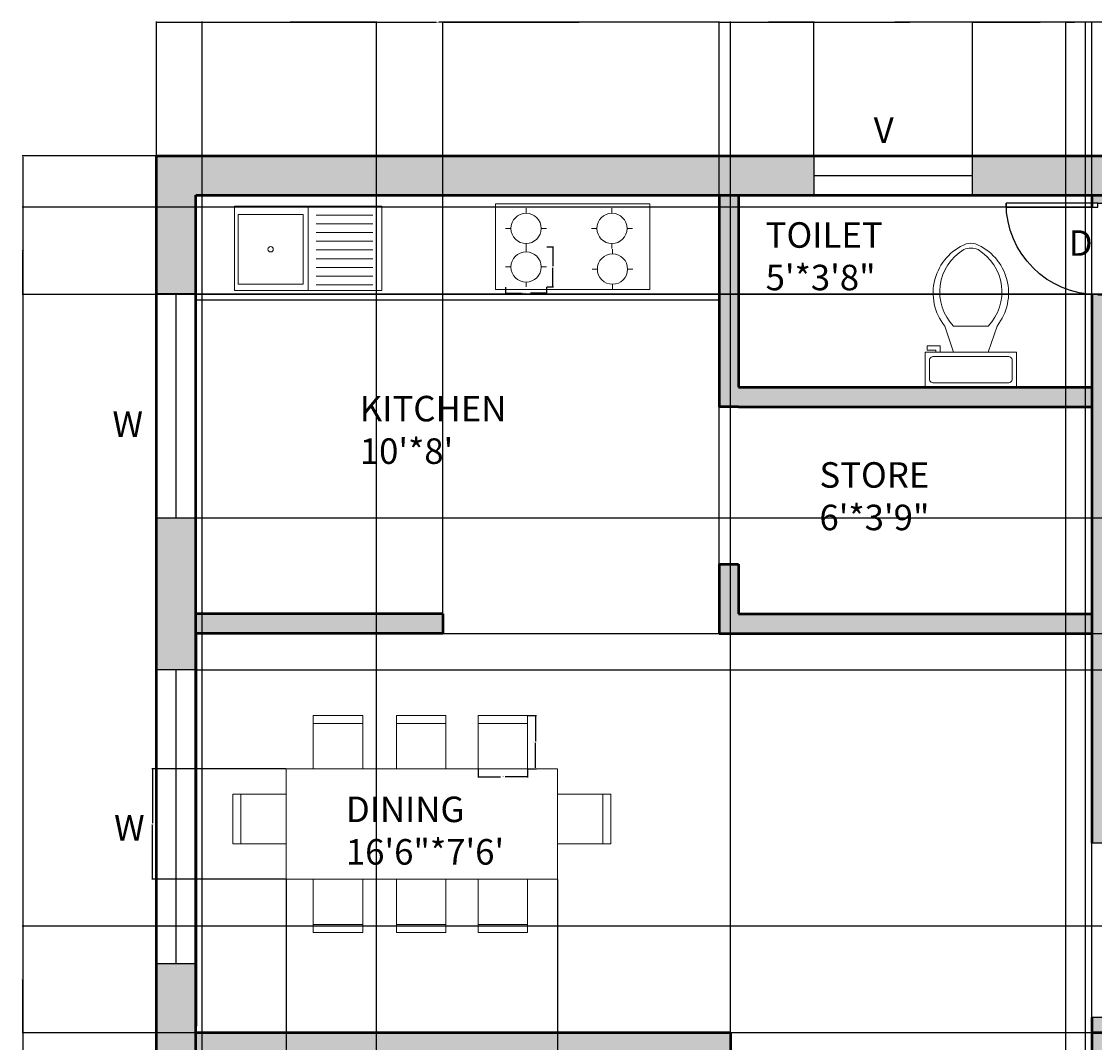
# Model space of a CAD drawing. Units: inches. Extents: x 678 to 1100, y 1432 to 2094.
# Tile 4 of 5: x 678 to 924, y 1860 to 2094. Entities that reach past the tile are written whole.
import ezdxf

# ---------------------------------------------------------------- set-up
doc = ezdxf.new("R2010")
doc.units = ezdxf.units.IN
for name, color, linetype, lineweight in [('A-ANNO-DIMS', 2, 'Continuous', 18), ('A-AREA-IDEN', 141, 'Continuous', 25), ('A-EQPM', 30, 'Continuous', 18), ('A-FLOR-CASE', 30, 'Continuous', 25), ('A-FLOR-FIXT', 9, 'Continuous', 18), ('A-WALL-PATT', 252, 'Continuous', 13), ('DOOR', 52, 'Continuous', 25), ('FUR', 30, 'Continuous', 18), ('TEXT', 141, 'Continuous', 18), ('WALL', 140, 'Continuous', 50), ('WIND', 212, 'Continuous', 25)]:
    doc.layers.add(name, color=color, linetype=linetype, lineweight=lineweight)
doc.styles.get("Standard").update_dxf_attribs({"font": 'arial.ttf'})
doc.dimstyles.get("Standard").update_dxf_attribs({"dimtxt": 0.18, "dimasz": 0.18, "dimexe": 0.18, "dimexo": 0.0625, "dimgap": 0.09, "dimtad": 0, "dimtih": 1, "dimtoh": 1, "dimdec": 4, "dimzin": 0, "dimdsep": 46, "dimtxsty": 'Standard', "dimcen": 0.09, "dimadec": 0, "dimazin": 0, "dimtfac": 1, "dimtdec": 4, "dimtofl": 0, "dimtmove": 0, "dimatfit": 3, "dimfxl": 1, "dimtolj": 1, "dimtzin": 0, "dimarcsym": 0})

# ---------------------------------------------------------------- blocks, each defined once
blk = doc.blocks.new('*U2')
for p, q in [((0, 0), (0, -6)), ((40, 0), (40, -6))]:
    blk.add_line(p, q)
blk.add_lwpolyline([(0, 0), (0, 40), (1.75, 40), (1.75, 0)], close=True)
blk.add_arc((0, 0), 40, 0, 90)
blk = doc.blocks.new('*U4')
for p, q in [((9.5, -6), (9.5, -2)), ((-10, -8.5), (-8, -8.5)), ((-10, -9.5), (-10, -8.5)), ((-7, -9.5), (-10, -9.5)), ((-8, -8.5), (-8, -8)), ((-7, -8), (-7, -9.5)), ((-4, -8), (-6, -14)), ((4, -8), (6, -14)), ((4, -14), (-4, -14))]:
    blk.add_line(p, q)
blk.add_lwpolyline([(10.5, -8), (10.5, 0), (-10.5, 0), (-10.5, -8)], close=True)
for points in [[(-9.5, -2), (-9.5, -6)], [(8.5, -1), (-8.5, -1)], [(-8.5, -7), (8.5, -7)]]:
    blk.add_lwpolyline(points)
for centre, radius, start, end in [((-8.62, -1.88), 0.884, 81.8699, 188.1301), ((8.62, -1.88), 0.884, 351.8699, 98.1301), ((-8.62, -6.12), 0.884, 171.8699, 278.1301), ((8.62, -6.12), 0.884, 261.8699, 8.1301), ((3.52, -21.58), 12.17, 141.4691, 247.9714), ((4.2, -21.82), 11.33, 136.3677, 238.9468), ((-3.52, -21.58), 12.17, 292.0284, 38.5307), ((-4.2, -21.82), 11.33, 301.053, 43.6321), ((0, -27.88), 4, 245.7318, 294.2682), ((0, -29), 4, 254.8605, 285.1395)]:
    blk.add_arc(centre, radius, start, end)
blk = doc.blocks.new('CHAIR-DINING')
blk.add_line((0, 10.39), (11.35, 10.39))
blk.add_lwpolyline([(0, 0), (11.35, 0), (11.35, 12.23), (0, 12.23)], close=True)
blk = doc.blocks.new('COOKTOP-BURNER')
for p, q in [((4.69, 8.04), (4.69, 9.18)), ((1.22, 4.57), (0, 4.57)), ((8.16, 4.57), (9.38, 4.57)), ((4.69, 1.1), (4.69, 0))]:
    blk.add_line(p, q)
blk.add_circle((4.69, 4.57), 3.47)
blk = doc.blocks.new('WIN-STANDARD')
blk.add_line((4.5, 0), (4.5, 67.31))
blk.add_lwpolyline([(9, 67.31), (0, 67.31), (0, 0), (9, 0)], close=True)
blk = doc.blocks.new('*D18')
at = {"layer": 'A-ANNO-DIMS', "color": 0, "lineweight": -2, "transparency": 16777216}
for p, q in [((794.13, 1934.68), (796.08, 1934.68)), ((795.9, 1934.5), (795.9, 1928.75)), ((795.9, 1922.64), (795.9, 1928.39)), ((794.13, 1922.46), (796.08, 1922.46))]:
    blk.add_line(p, q, dxfattribs=at)
at = {"layer": 'A-ANNO-DIMS', "color": 0, "transparency": 16777216}
for points in [[(795.87, 1934.5), (795.93, 1934.5), (795.9, 1934.68)], [(795.87, 1922.64), (795.93, 1922.64), (795.9, 1922.46)]]:
    blk.add_solid(points, dxfattribs=at)
at = {"layer": 'Defpoints', "color": 0, "transparency": 16777216}
for p in [(794.06, 1934.68), (795.9, 1934.68), (794.06, 1922.46)]:
    blk.add_point(p, dxfattribs=at)
at = {"layer": 'A-ANNO-DIMS', "color": 0, "transparency": 16777216, "insert": (795.9, 1928.57), "char_height": 0.18, "attachment_point": 5}
blk.add_mtext('\\A1;CHAIR 12 TYP.', dxfattribs=at)
blk = doc.blocks.new('*D19')
at = {"layer": 'A-ANNO-DIMS', "color": 0, "lineweight": -2, "transparency": 16777216}
for p, q in [((782.71, 1922.39), (782.71, 1920.44)), ((794.06, 1922.39), (794.06, 1920.44)), ((782.89, 1920.62), (787.87, 1920.62)), ((793.88, 1920.62), (788.91, 1920.62))]:
    blk.add_line(p, q, dxfattribs=at)
at = {"layer": 'A-ANNO-DIMS', "color": 0, "transparency": 16777216}
for points in [[(782.89, 1920.65), (782.89, 1920.59), (782.71, 1920.62)], [(793.88, 1920.65), (793.88, 1920.59), (794.06, 1920.62)]]:
    blk.add_solid(points, dxfattribs=at)
at = {"layer": 'Defpoints', "color": 0, "transparency": 16777216}
for p in [(782.71, 1922.46), (794.06, 1922.46), (794.06, 1920.62)]:
    blk.add_point(p, dxfattribs=at)
at = {"layer": 'A-ANNO-DIMS', "color": 0, "transparency": 16777216, "insert": (788.39, 1920.62), "char_height": 0.18, "attachment_point": 5}
blk.add_mtext('\\A1;11 TYP.', dxfattribs=at)
blk = doc.blocks.new('*D22')
at = {"layer": 'A-ANNO-DIMS', "color": 0, "lineweight": -2, "transparency": 16777216}
for p, q in [((789.03, 2032.84), (789.03, 2031.31)), ((798.41, 2032.84), (798.41, 2031.31)), ((789.21, 2031.49), (792.7, 2031.49)), ((798.23, 2031.49), (794.74, 2031.49))]:
    blk.add_line(p, q, dxfattribs=at)
at = {"layer": 'A-ANNO-DIMS', "color": 0, "transparency": 16777216}
for points in [[(789.21, 2031.52), (789.21, 2031.46), (789.03, 2031.49)], [(798.23, 2031.52), (798.23, 2031.46), (798.41, 2031.49)]]:
    blk.add_solid(points, dxfattribs=at)
at = {"layer": 'Defpoints', "color": 0, "transparency": 16777216}
for p in [(789.03, 2032.9), (798.41, 2032.9), (798.41, 2031.49)]:
    blk.add_point(p, dxfattribs=at)
at = {"layer": 'A-ANNO-DIMS', "color": 0, "transparency": 16777216, "insert": (793.72, 2031.49), "char_height": 0.18, "attachment_point": 5}
blk.add_mtext('\\A1;BURNER 9 TYP.', dxfattribs=at)
blk = doc.blocks.new('*D23')
at = {"layer": 'A-ANNO-DIMS', "color": 0, "lineweight": -2, "transparency": 16777216}
for p, q in [((798.47, 2042.08), (800, 2042.08)), ((799.82, 2041.9), (799.82, 2037.67)), ((799.82, 2033.08), (799.82, 2037.31)), ((798.47, 2032.9), (800, 2032.9))]:
    blk.add_line(p, q, dxfattribs=at)
at = {"layer": 'A-ANNO-DIMS', "color": 0, "transparency": 16777216}
for points in [[(799.79, 2041.9), (799.85, 2041.9), (799.82, 2042.08)], [(799.79, 2033.08), (799.85, 2033.08), (799.82, 2032.9)]]:
    blk.add_solid(points, dxfattribs=at)
at = {"layer": 'Defpoints', "color": 0, "transparency": 16777216}
for p in [(798.41, 2042.08), (799.82, 2042.08), (798.41, 2032.9)]:
    blk.add_point(p, dxfattribs=at)
at = {"layer": 'A-ANNO-DIMS', "color": 0, "transparency": 16777216, "insert": (799.82, 2037.49), "char_height": 0.18, "attachment_point": 5}
blk.add_mtext('\\A1;9 TYP.', dxfattribs=at)
blk = doc.blocks.new('*D25')
at = {"layer": 'A-ANNO-DIMS', "color": 0, "lineweight": -2, "transparency": 16777216}
for p, q in [((708.9, 2062.93), (678.13, 2062.93)), ((678.31, 2062.75), (678.31, 1763.11)), ((678.31, 1463.11), (678.31, 1762.75)), ((708.9, 1462.93), (678.13, 1462.93))]:
    blk.add_line(p, q, dxfattribs=at)
at = {"layer": 'A-ANNO-DIMS', "color": 0, "transparency": 16777216}
for points in [[(678.28, 2062.75), (678.34, 2062.75), (678.31, 2062.93)], [(678.28, 1463.11), (678.34, 1463.11), (678.31, 1462.93)]]:
    blk.add_solid(points, dxfattribs=at)
at = {"layer": 'Defpoints', "color": 0, "transparency": 16777216}
for p in [(678.31, 2062.93), (708.96, 2062.93), (708.96, 1462.93)]:
    blk.add_point(p, dxfattribs=at)
at = {"layer": 'A-ANNO-DIMS', "color": 0, "transparency": 16777216, "insert": (678.31, 1762.93), "char_height": 0.18, "attachment_point": 5}
blk.add_mtext('\\A1;600', dxfattribs=at)
blk = doc.blocks.new('*D26')
at = {"layer": 'A-ANNO-DIMS', "color": 0, "lineweight": -2, "transparency": 16777216}
for p, q in [((708.96, 2062.99), (708.96, 2093.76)), ((709.14, 2093.58), (773.18, 2093.58)), ((837.78, 2093.58), (773.74, 2093.58)), ((837.96, 2053.99), (837.96, 2093.76))]:
    blk.add_line(p, q, dxfattribs=at)
at = {"layer": 'A-ANNO-DIMS', "color": 0, "transparency": 16777216}
for points in [[(709.14, 2093.61), (709.14, 2093.55), (708.96, 2093.58)], [(837.78, 2093.61), (837.78, 2093.55), (837.96, 2093.58)]]:
    blk.add_solid(points, dxfattribs=at)
at = {"layer": 'Defpoints', "color": 0, "transparency": 16777216}
for p in [(837.96, 2093.58), (708.96, 2062.93), (837.96, 2053.93)]:
    blk.add_point(p, dxfattribs=at)
at = {"layer": 'A-ANNO-DIMS', "color": 0, "transparency": 16777216, "insert": (773.46, 2093.58), "char_height": 0.18, "attachment_point": 5}
blk.add_mtext('\\A1;129', dxfattribs=at)
blk = doc.blocks.new('*D27')
at = {"layer": 'A-ANNO-DIMS', "color": 0, "lineweight": -2, "transparency": 16777216}
for p, q in [((837.96, 2053.99), (837.96, 2093.76)), ((838.14, 2093.58), (848.37, 2093.58)), ((859.53, 2093.58), (849.3, 2093.58)), ((859.71, 2062.99), (859.71, 2093.76))]:
    blk.add_line(p, q, dxfattribs=at)
at = {"layer": 'A-ANNO-DIMS', "color": 0, "transparency": 16777216}
for points in [[(838.14, 2093.61), (838.14, 2093.55), (837.96, 2093.58)], [(859.53, 2093.61), (859.53, 2093.55), (859.71, 2093.58)]]:
    blk.add_solid(points, dxfattribs=at)
at = {"layer": 'Defpoints', "color": 0, "transparency": 16777216}
for p in [(859.71, 2093.58), (859.71, 2062.93), (837.96, 2053.93)]:
    blk.add_point(p, dxfattribs=at)
at = {"layer": 'A-ANNO-DIMS', "color": 0, "transparency": 16777216, "insert": (848.84, 2093.58), "char_height": 0.18, "attachment_point": 5}
blk.add_mtext('\\A1;21.753', dxfattribs=at)
blk = doc.blocks.new('*D28')
at = {"layer": 'A-ANNO-DIMS', "color": 0, "lineweight": -2, "transparency": 16777216}
for p, q in [((859.71, 2062.99), (859.71, 2093.76)), ((859.89, 2093.58), (877.5, 2093.58)), ((895.89, 2093.58), (878.29, 2093.58)), ((896.07, 2062.99), (896.07, 2093.76))]:
    blk.add_line(p, q, dxfattribs=at)
at = {"layer": 'A-ANNO-DIMS', "color": 0, "transparency": 16777216}
for points in [[(859.89, 2093.61), (859.89, 2093.55), (859.71, 2093.58)], [(895.89, 2093.61), (895.89, 2093.55), (896.07, 2093.58)]]:
    blk.add_solid(points, dxfattribs=at)
at = {"layer": 'Defpoints', "color": 0, "transparency": 16777216}
for p in [(896.07, 2093.58), (859.71, 2062.93), (896.07, 2062.93)]:
    blk.add_point(p, dxfattribs=at)
at = {"layer": 'A-ANNO-DIMS', "color": 0, "transparency": 16777216, "insert": (877.89, 2093.58), "char_height": 0.18, "attachment_point": 5}
blk.add_mtext('\\A1;36.36', dxfattribs=at)
blk = doc.blocks.new('*D29')
at = {"layer": 'A-ANNO-DIMS', "color": 0, "lineweight": -2, "transparency": 16777216}
for p, q in [((896.07, 2062.99), (896.07, 2093.76)), ((896.25, 2093.58), (911.62, 2093.58)), ((927.78, 2093.58), (912.41, 2093.58)), ((927.96, 2053.99), (927.96, 2093.76))]:
    blk.add_line(p, q, dxfattribs=at)
at = {"layer": 'A-ANNO-DIMS', "color": 0, "transparency": 16777216}
for points in [[(896.25, 2093.61), (896.25, 2093.55), (896.07, 2093.58)], [(927.78, 2093.61), (927.78, 2093.55), (927.96, 2093.58)]]:
    blk.add_solid(points, dxfattribs=at)
at = {"layer": 'Defpoints', "color": 0, "transparency": 16777216}
for p in [(927.96, 2093.58), (896.07, 2062.93), (927.96, 2053.93)]:
    blk.add_point(p, dxfattribs=at)
at = {"layer": 'A-ANNO-DIMS', "color": 0, "transparency": 16777216, "insert": (912.02, 2093.58), "char_height": 0.18, "attachment_point": 5}
blk.add_mtext('\\A1;31.89', dxfattribs=at)
blk = doc.blocks.new('*D42')
at = {"layer": 'A-ANNO-DIMS', "color": 0, "lineweight": -2, "transparency": 16777216}
for p, q in [((718.02, 1953.43), (1099.79, 1953.43)), ((1099.61, 1953.25), (1099.61, 1949.47)), ((1099.61, 1945.33), (1099.61, 1949.11)), ((718.02, 1945.15), (1099.79, 1945.15))]:
    blk.add_line(p, q, dxfattribs=at)
at = {"layer": 'A-ANNO-DIMS', "color": 0, "transparency": 16777216}
for points in [[(1099.58, 1953.25), (1099.64, 1953.25), (1099.61, 1953.43)], [(1099.58, 1945.33), (1099.64, 1945.33), (1099.61, 1945.15)]]:
    blk.add_solid(points, dxfattribs=at)
at = {"layer": 'Defpoints', "color": 0, "transparency": 16777216}
for p in [(717.96, 1953.43), (1099.61, 1953.43), (717.96, 1945.15)]:
    blk.add_point(p, dxfattribs=at)
at = {"layer": 'A-ANNO-DIMS', "color": 0, "transparency": 16777216, "insert": (1099.61, 1949.29), "char_height": 0.18, "attachment_point": 5}
blk.add_mtext('\\A1;8.282', dxfattribs=at)
blk = doc.blocks.new('*D43')
at = {"layer": 'A-ANNO-DIMS', "color": 0, "lineweight": -2, "transparency": 16777216}
for p, q in [((718.02, 2031.32), (1099.79, 2031.32)), ((1099.61, 2031.14), (1099.61, 2005.81)), ((1099.61, 1980.12), (1099.61, 2005.45)), ((718.02, 1979.94), (1099.79, 1979.94))]:
    blk.add_line(p, q, dxfattribs=at)
at = {"layer": 'A-ANNO-DIMS', "color": 0, "transparency": 16777216}
for points in [[(1099.58, 2031.14), (1099.64, 2031.14), (1099.61, 2031.32)], [(1099.58, 1980.12), (1099.64, 1980.12), (1099.61, 1979.94)]]:
    blk.add_solid(points, dxfattribs=at)
at = {"layer": 'Defpoints', "color": 0, "transparency": 16777216}
for p in [(717.96, 2031.32), (1099.61, 2031.32), (717.96, 1979.94)]:
    blk.add_point(p, dxfattribs=at)
at = {"layer": 'A-ANNO-DIMS', "color": 0, "transparency": 16777216, "insert": (1099.61, 2005.63), "char_height": 0.18, "attachment_point": 5}
blk.add_mtext('\\A1;51.38', dxfattribs=at)
blk = doc.blocks.new('*D44')
at = {"layer": 'A-ANNO-DIMS', "color": 0, "lineweight": -2, "transparency": 16777216}
for p, q in [((718.02, 2053.93), (1099.79, 2053.93)), ((1099.61, 2053.75), (1099.61, 2042.81)), ((1099.61, 2031.5), (1099.61, 2042.44)), ((718.02, 2031.32), (1099.79, 2031.32))]:
    blk.add_line(p, q, dxfattribs=at)
at = {"layer": 'A-ANNO-DIMS', "color": 0, "transparency": 16777216}
for points in [[(1099.58, 2053.75), (1099.64, 2053.75), (1099.61, 2053.93)], [(1099.58, 2031.5), (1099.64, 2031.5), (1099.61, 2031.32)]]:
    blk.add_solid(points, dxfattribs=at)
at = {"layer": 'Defpoints', "color": 0, "transparency": 16777216}
for p in [(717.96, 2053.93), (1099.61, 2053.93), (717.96, 2031.32)]:
    blk.add_point(p, dxfattribs=at)
at = {"layer": 'A-ANNO-DIMS', "color": 0, "transparency": 16777216, "insert": (1099.61, 2042.62), "char_height": 0.18, "attachment_point": 5}
blk.add_mtext('\\A1;22.61', dxfattribs=at)
blk = doc.blocks.new('*D45')
at = {"layer": 'A-ANNO-DIMS', "color": 0, "lineweight": -2, "transparency": 16777216}
for p, q in [((719.41, 1684.99), (719.41, 2093.76)), ((719.59, 2093.58), (739.19, 2093.58)), ((759.23, 2093.58), (739.63, 2093.58)), ((759.41, 1684.99), (759.41, 2093.76))]:
    blk.add_line(p, q, dxfattribs=at)
at = {"layer": 'A-ANNO-DIMS', "color": 0, "transparency": 16777216}
for points in [[(719.59, 2093.61), (719.59, 2093.55), (719.41, 2093.58)], [(759.23, 2093.61), (759.23, 2093.55), (759.41, 2093.58)]]:
    blk.add_solid(points, dxfattribs=at)
at = {"layer": 'Defpoints', "color": 0, "transparency": 16777216}
for p in [(759.41, 2093.58), (719.41, 1684.93), (759.41, 1684.93)]:
    blk.add_point(p, dxfattribs=at)
at = {"layer": 'A-ANNO-DIMS', "color": 0, "transparency": 16777216, "insert": (739.41, 2093.58), "char_height": 0.18, "attachment_point": 5}
blk.add_mtext('\\A1;40', dxfattribs=at)
blk = doc.blocks.new('*D47')
at = {"layer": 'A-ANNO-DIMS', "color": 0, "lineweight": -2, "transparency": 16777216}
for p, q in [((923.4, 2051.21), (678.13, 2051.21)), ((678.31, 2051.03), (678.31, 2041.37)), ((678.31, 2031.35), (678.31, 2041.01)), ((923.4, 2031.17), (678.13, 2031.17))]:
    blk.add_line(p, q, dxfattribs=at)
at = {"layer": 'A-ANNO-DIMS', "color": 0, "transparency": 16777216}
for points in [[(678.28, 2051.03), (678.34, 2051.03), (678.31, 2051.21)], [(678.28, 2031.35), (678.34, 2031.35), (678.31, 2031.17)]]:
    blk.add_solid(points, dxfattribs=at)
at = {"layer": 'Defpoints', "color": 0, "transparency": 16777216}
for p in [(678.31, 2051.21), (923.46, 2051.21), (923.46, 2031.17)]:
    blk.add_point(p, dxfattribs=at)
at = {"layer": 'A-ANNO-DIMS', "color": 0, "transparency": 16777216, "insert": (678.31, 2041.19), "char_height": 0.18, "attachment_point": 5}
blk.add_mtext('\\A1;20.04', dxfattribs=at)
blk = doc.blocks.new('*D48')
at = {"layer": 'A-ANNO-DIMS', "color": 0, "lineweight": -2, "transparency": 16777216}
for p, q in [((917.46, 1560.49), (917.46, 2093.76)), ((917.64, 2093.58), (919.45, 2093.58)), ((921.78, 2093.58), (919.97, 2093.58)), ((921.96, 1560.49), (921.96, 2093.76))]:
    blk.add_line(p, q, dxfattribs=at)
at = {"layer": 'A-ANNO-DIMS', "color": 0, "transparency": 16777216}
for points in [[(917.64, 2093.61), (917.64, 2093.55), (917.46, 2093.58)], [(921.78, 2093.61), (921.78, 2093.55), (921.96, 2093.58)]]:
    blk.add_solid(points, dxfattribs=at)
at = {"layer": 'Defpoints', "color": 0, "transparency": 16777216}
for p in [(921.96, 2093.58), (917.46, 1560.43), (921.96, 1560.43)]:
    blk.add_point(p, dxfattribs=at)
at = {"layer": 'A-ANNO-DIMS', "color": 0, "transparency": 16777216, "insert": (919.71, 2093.58), "char_height": 0.18, "attachment_point": 5}
blk.add_mtext('\\A1;4.5', dxfattribs=at)
blk = doc.blocks.new('*D51')
at = {"layer": 'A-ANNO-DIMS', "color": 0, "lineweight": -2, "transparency": 16777216}
for p, q in [((774.64, 1957.99), (774.64, 2093.76)), ((774.82, 2093.58), (805.9, 2093.58)), ((837.78, 2093.58), (806.69, 2093.58)), ((837.96, 1953.49), (837.96, 2093.76))]:
    blk.add_line(p, q, dxfattribs=at)
at = {"layer": 'A-ANNO-DIMS', "color": 0, "transparency": 16777216}
for points in [[(774.82, 2093.61), (774.82, 2093.55), (774.64, 2093.58)], [(837.78, 2093.61), (837.78, 2093.55), (837.96, 2093.58)]]:
    blk.add_solid(points, dxfattribs=at)
at = {"layer": 'Defpoints', "color": 0, "transparency": 16777216}
for p in [(837.96, 2093.58), (774.64, 1957.93), (837.96, 1953.43)]:
    blk.add_point(p, dxfattribs=at)
at = {"layer": 'A-ANNO-DIMS', "color": 0, "transparency": 16777216, "insert": (806.3, 2093.58), "char_height": 0.18, "attachment_point": 5}
blk.add_mtext('\\A1;63.32', dxfattribs=at)
blk = doc.blocks.new('*D52')
at = {"layer": 'A-ANNO-DIMS', "color": 0, "lineweight": -2, "transparency": 16777216}
for p, q in [((840.56, 1861.99), (840.56, 2093.76)), ((840.74, 2093.58), (881.69, 2093.58)), ((923.28, 2093.58), (882.33, 2093.58)), ((923.46, 1861.99), (923.46, 2093.76))]:
    blk.add_line(p, q, dxfattribs=at)
at = {"layer": 'A-ANNO-DIMS', "color": 0, "transparency": 16777216}
for points in [[(840.74, 2093.61), (840.74, 2093.55), (840.56, 2093.58)], [(923.28, 2093.61), (923.28, 2093.55), (923.46, 2093.58)]]:
    blk.add_solid(points, dxfattribs=at)
at = {"layer": 'Defpoints', "color": 0, "transparency": 16777216}
for p in [(923.46, 2093.58), (840.56, 1861.93), (923.46, 1861.93)]:
    blk.add_point(p, dxfattribs=at)
at = {"layer": 'A-ANNO-DIMS', "color": 0, "transparency": 16777216, "insert": (882.01, 2093.58), "char_height": 0.18, "attachment_point": 5}
blk.add_mtext('\\A1;82.9', dxfattribs=at)
blk = doc.blocks.new('*D53')
at = {"layer": 'A-ANNO-DIMS', "color": 0, "lineweight": -2, "transparency": 16777216}
for p, q in [((738.71, 1897.06), (738.71, 1432.1)), ((800.95, 1897.06), (800.95, 1432.1)), ((738.89, 1432.28), (769.43, 1432.28)), ((800.77, 1432.28), (770.22, 1432.28))]:
    blk.add_line(p, q, dxfattribs=at)
at = {"layer": 'A-ANNO-DIMS', "color": 0, "transparency": 16777216}
for points in [[(738.89, 1432.31), (738.89, 1432.25), (738.71, 1432.28)], [(800.77, 1432.31), (800.77, 1432.25), (800.95, 1432.28)]]:
    blk.add_solid(points, dxfattribs=at)
at = {"layer": 'Defpoints', "color": 0, "transparency": 16777216}
for p in [(738.71, 1897.12), (800.95, 1897.12), (800.95, 1432.28)]:
    blk.add_point(p, dxfattribs=at)
at = {"layer": 'A-ANNO-DIMS', "color": 0, "transparency": 16777216, "insert": (769.83, 1432.28), "char_height": 0.18, "attachment_point": 5}
blk.add_mtext('\\A1;62.25', dxfattribs=at)
blk = doc.blocks.new('*D54')
at = {"layer": 'A-ANNO-DIMS', "color": 0, "lineweight": -2, "transparency": 16777216}
for p, q in [((738.64, 1922.46), (707.88, 1922.46)), ((708.06, 1922.28), (708.06, 1909.97)), ((708.06, 1897.3), (708.06, 1909.61)), ((738.64, 1897.12), (707.88, 1897.12))]:
    blk.add_line(p, q, dxfattribs=at)
at = {"layer": 'A-ANNO-DIMS', "color": 0, "transparency": 16777216}
for points in [[(708.03, 1922.28), (708.09, 1922.28), (708.06, 1922.46)], [(708.03, 1897.3), (708.09, 1897.3), (708.06, 1897.12)]]:
    blk.add_solid(points, dxfattribs=at)
at = {"layer": 'Defpoints', "color": 0, "transparency": 16777216}
for p in [(708.06, 1922.46), (738.71, 1922.46), (738.71, 1897.12)]:
    blk.add_point(p, dxfattribs=at)
at = {"layer": 'A-ANNO-DIMS', "color": 0, "transparency": 16777216, "insert": (708.06, 1909.79), "char_height": 0.18, "attachment_point": 5}
blk.add_mtext('\\A1;25.337', dxfattribs=at)
blk = doc.blocks.new('*D58')
at = {"layer": 'A-ANNO-DIMS', "color": 0, "lineweight": -2, "transparency": 16777216}
for p, q in [((996.9, 1886.38), (678.13, 1886.38)), ((678.31, 1886.2), (678.31, 1874.34)), ((678.31, 1862.11), (678.31, 1873.97)), ((996.9, 1861.93), (678.13, 1861.93))]:
    blk.add_line(p, q, dxfattribs=at)
at = {"layer": 'A-ANNO-DIMS', "color": 0, "transparency": 16777216}
for points in [[(678.28, 1886.2), (678.34, 1886.2), (678.31, 1886.38)], [(678.28, 1862.11), (678.34, 1862.11), (678.31, 1861.93)]]:
    blk.add_solid(points, dxfattribs=at)
at = {"layer": 'Defpoints', "color": 0, "transparency": 16777216}
for p in [(678.31, 1886.38), (996.96, 1886.38), (996.96, 1861.93)]:
    blk.add_point(p, dxfattribs=at)
at = {"layer": 'A-ANNO-DIMS', "color": 0, "transparency": 16777216, "insert": (678.31, 1874.15), "char_height": 0.18, "attachment_point": 5}
blk.add_mtext('\\A1;24.45', dxfattribs=at)

msp = doc.modelspace()

# ---------------------------------------------------------------- hatches: boundary and pattern name
at = {"layer": 'A-WALL-PATT'}
h = msp.add_hatch(color=256, dxfattribs=at)
h.dxf.hatch_style = 1
h.paths.add_polyline_path([(859.7133, 2062.9286), (708.9606, 2062.9286), (708.9606, 2031.3203), (717.9606, 2031.3203), (717.9606, 2053.9286), (837.9606, 2053.9286), (859.7133, 2053.9286)])
h.paths.add_polyline_path([(957.0069, 2062.9286), (896.0724, 2062.9286), (896.0724, 2053.9286), (957.0069, 2053.9286)])
h.paths.add_polyline_path([(842.4606, 2053.9286), (837.9606, 2053.9286), (837.9606, 2005.4286), (842.4606, 2005.4286), (923.4606, 2005.4286), (923.4606, 2009.9286), (842.4606, 2009.9286)])
h.paths.add_polyline_path([(927.9606, 2053.9286), (923.4606, 2053.9286), (923.4606, 2052.1286), (924.8103, 2052.1286), (927.9606, 2052.1286)])
h.paths.add_polyline_path([(1068.9606, 2062.9286), (1024.3184, 2062.9286), (1024.3184, 2053.9286), (1028.6041, 2053.9286), (1059.9606, 2053.9286), (1059.9606, 2002.6361), (1068.9606, 2002.6361)])
h.paths.add_polyline_path([(1059.9606, 1861.9286), (996.9604, 1861.9286), (927.9606, 1861.9286), (923.4606, 1861.9286), (923.4606, 1857.4286), (1059.9606, 1857.4286)], flags=17)
h.paths.add_polyline_path([(927.9606, 2031.1269), (924.8103, 2031.1269, -0.01607952), (923.4606, 2031.1703), (923.4606, 1905.3856), (927.9606, 1905.3856)])
h.paths.add_polyline_path([(923.4606, 1957.9286), (842.4606, 1957.9286), (842.4606, 1969.339), (837.9606, 1969.339), (837.9606, 1953.4286), (923.4606, 1953.4286)])
h.paths.add_polyline_path([(774.6357, 1957.9286), (717.9606, 1957.9286), (717.9606, 1953.4286), (774.6357, 1953.4286)])
h.paths.add_polyline_path([(717.9606, 1979.9404), (708.9606, 1979.9404), (708.9606, 1945.1463), (717.9606, 1945.1463)])
h.paths.add_polyline_path([(840.5596, 1861.9286), (717.9606, 1861.9286), (717.9606, 1857.4286), (840.5596, 1857.4286)], flags=17)
h.paths.add_polyline_path([(927.9606, 1865.3856), (923.4606, 1865.3856), (923.4606, 1861.9286), (927.9606, 1861.9286)], flags=17)
h.paths.add_polyline_path([(1059.9606, 1689.4286), (967.3461, 1689.4286), (967.3461, 1684.9286), (1059.9606, 1684.9286)], flags=17)
h.paths.add_polyline_path([(987.9606, 1737.4286), (983.4606, 1737.4286), (983.4606, 1715.196), (986.7357, 1715.196, -0.01403382), (987.9606, 1715.1616)], flags=17)
h.paths.add_polyline_path([(916.0499, 2036.8414), (924.8721, 2036.8414), (924.8721, 2048.8901), (916.0499, 2048.8901)], flags=9)
h.paths.add_polyline_path([(921.7778, 1883.2914), (930.5999, 1883.2914), (930.5999, 1895.3401), (921.7778, 1895.3401)], flags=25)
h.paths.add_polyline_path([(732.1085, 1683.0506), (740.9307, 1683.0506), (740.9307, 1695.0993), (732.1085, 1695.0993)], flags=25)
h.paths.add_polyline_path([(943.8458, 1737.5114), (952.6679, 1737.5114), (952.6679, 1749.5601), (943.8458, 1749.5601)], flags=25)
h.paths.add_polyline_path([(986.0751, 1696.9795), (994.8973, 1696.9795), (994.8973, 1709.0282), (986.0751, 1709.0282)], flags=25)
h.paths.add_polyline_path([(940.1881, 1677.378), (949.0103, 1677.378), (949.0103, 1689.4267), (940.1881, 1689.4267)], flags=25)
h.paths.add_polyline_path([(998.6262, 1761.7469), (1044.0453, 1761.7469), (1044.0453, 1783.5644), (998.6262, 1783.5644)], flags=25)
h.paths.add_polyline_path([(997.3001, 1713.4735), (1028.9316, 1713.4735), (1028.9316, 1735.2909), (997.3001, 1735.2909)], flags=25)
h.paths.add_polyline_path([(1005.9896, 1586.8139), (1051.4087, 1586.8139), (1051.4087, 1608.6313), (1005.9896, 1608.6313)], flags=25)
h.paths.add_polyline_path([(794.7038, 1552.8124), (873.8721, 1552.8124), (873.8721, 1574.6298), (794.7038, 1574.6298)], flags=25)
h.paths.add_polyline_path([(774.2693, 1771.1228), (831.9444, 1771.1228), (831.9444, 1792.9403), (774.2693, 1792.9403)], flags=25)
h.paths.add_polyline_path([(750.0357, 1897.1514), (786.4291, 1897.1514), (786.4291, 1918.9689), (750.0357, 1918.9689)], flags=25)
h.paths.add_polyline_path([(974.9086, 1953.7921), (1020.3276, 1953.7921), (1020.3276, 1975.6096), (974.9086, 1975.6096)], flags=9)
h.paths.add_polyline_path([(859.1564, 1973.8092), (890.2175, 1973.8092), (890.2175, 1995.6267), (859.1564, 1995.6267)], flags=9)
h.paths.add_polyline_path([(753.2305, 1989.0219), (792.2962, 1989.0219), (792.2962, 2010.8393), (753.2305, 2010.8393)], flags=9)
h.paths.add_polyline_path([(1067.3992, 1620.1515), (1078.032, 1620.1515), (1078.032, 1632.2002), (1067.3992, 1632.2002)], flags=9)
h.paths.add_polyline_path([(846.8446, 2028.8178), (878.5079, 2028.8178), (878.5079, 2050.6353), (846.8446, 2050.6353)], flags=25)
h.paths.add_polyline_path([(1059.9606, 1832.7202), (1068.9606, 1832.7202), (1068.9606, 1935.3246), (1059.9606, 1935.3246)])
h.paths.add_polyline_path([(1068.9606, 1765.4088), (1059.9606, 1765.4088), (1059.9606, 1728.1446), (1068.9606, 1728.1446)])
h.paths.add_polyline_path([(1059.9606, 1657.7018), (1068.9606, 1657.7018), (1068.9606, 1697.8017), (1059.9606, 1697.8017)])
h.paths.add_polyline_path([(1068.9606, 1590.3903), (1059.9606, 1590.3903), (1059.9606, 1551.1623), (1068.9606, 1551.1623)])
h.paths.add_polyline_path([(708.9606, 1826.8331), (717.9606, 1826.8331), (717.9606, 1877.8348), (708.9606, 1877.8348)])
h.paths.add_polyline_path([(717.9606, 1759.5217), (708.9606, 1759.5217), (708.9606, 1462.9286), (1068.9606, 1462.9286), (1068.9606, 1483.8508), (1059.9606, 1483.8508), (1059.9606, 1471.9286), (717.9606, 1471.9286)])
h = msp.add_hatch(color=256, dxfattribs=at)
h.dxf.hatch_style = 1
h.paths.add_polyline_path([(1059.9606, 1741.9286), (970.7942, 1741.9286), (970.7942, 1737.4286), (1059.9606, 1737.4286)])
h.paths.add_polyline_path([(927.3461, 1689.4286), (759.4099, 1689.4286), (759.4099, 1684.9286), (927.3461, 1684.9286)])
h.paths.add_polyline_path([(921.9606, 1684.9286), (917.4606, 1684.9286), (917.4606, 1560.4286), (921.9606, 1560.4286)])
h.paths.add_polyline_path([(1059.9606, 1564.9286), (921.9606, 1564.9286), (921.9606, 1560.4286), (1059.9606, 1560.4286)])
h.paths.add_polyline_path([(916.0499, 2036.8414), (924.8721, 2036.8414), (924.8721, 2048.8901), (916.0499, 2048.8901)], flags=9)
h.paths.add_polyline_path([(921.7778, 1883.2914), (930.5999, 1883.2914), (930.5999, 1895.3401), (921.7778, 1895.3401)], flags=9)
h.paths.add_polyline_path([(732.1085, 1683.0506), (740.9307, 1683.0506), (740.9307, 1695.0993), (732.1085, 1695.0993)], flags=9)
h.paths.add_polyline_path([(943.8458, 1737.5114), (952.6679, 1737.5114), (952.6679, 1749.5601), (943.8458, 1749.5601)], flags=9)
h.paths.add_polyline_path([(986.0751, 1696.9795), (994.8973, 1696.9795), (994.8973, 1709.0282), (986.0751, 1709.0282)], flags=9)
h.paths.add_polyline_path([(940.1881, 1677.378), (949.0103, 1677.378), (949.0103, 1689.4267), (940.1881, 1689.4267)], flags=9)
h.paths.add_polyline_path([(998.6262, 1761.7469), (1044.0453, 1761.7469), (1044.0453, 1783.5644), (998.6262, 1783.5644)], flags=9)
h.paths.add_polyline_path([(1005.9896, 1586.8139), (1051.4087, 1586.8139), (1051.4087, 1608.6313), (1005.9896, 1608.6313)], flags=9)
h.paths.add_polyline_path([(794.7038, 1552.8124), (873.8721, 1552.8124), (873.8721, 1574.6298), (794.7038, 1574.6298)], flags=9)
h.paths.add_polyline_path([(774.2693, 1771.1228), (831.9444, 1771.1228), (831.9444, 1792.9403), (774.2693, 1792.9403)], flags=9)
h.paths.add_polyline_path([(750.0357, 1897.1514), (786.4291, 1897.1514), (786.4291, 1918.9689), (750.0357, 1918.9689)], flags=9)
h.paths.add_polyline_path([(974.9086, 1953.7921), (1020.3276, 1953.7921), (1020.3276, 1975.6096), (974.9086, 1975.6096)], flags=9)
h.paths.add_polyline_path([(859.1564, 1973.8092), (890.2175, 1973.8092), (890.2175, 1995.6267), (859.1564, 1995.6267)], flags=9)
h.paths.add_polyline_path([(846.8446, 2028.8178), (878.5079, 2028.8178), (878.5079, 2050.6353), (846.8446, 2050.6353)], flags=9)
h.paths.add_polyline_path([(753.2305, 1989.0219), (792.2962, 1989.0219), (792.2962, 2010.8393), (753.2305, 2010.8393)], flags=9)
h = msp.add_hatch(color=256, dxfattribs=at)
h.dxf.hatch_style = 1
h.paths.add_polyline_path([(927.9606, 1857.4286), (923.4606, 1857.4286), (923.4606, 1737.4286), (927.9606, 1737.4286)])
h.paths.add_polyline_path([(930.7942, 1741.9286), (927.9606, 1741.9286), (927.9606, 1737.4286), (930.7942, 1737.4286)])
h.paths.add_polyline_path([(916.0499, 2036.8414), (924.8721, 2036.8414), (924.8721, 2048.8901), (916.0499, 2048.8901)], flags=9)
h.paths.add_polyline_path([(921.7778, 1883.2914), (930.5999, 1883.2914), (930.5999, 1895.3401), (921.7778, 1895.3401)], flags=9)
h.paths.add_polyline_path([(732.1085, 1683.0506), (740.9307, 1683.0506), (740.9307, 1695.0993), (732.1085, 1695.0993)], flags=9)
h.paths.add_polyline_path([(943.8458, 1737.5114), (952.6679, 1737.5114), (952.6679, 1749.5601), (943.8458, 1749.5601)], flags=9)
h.paths.add_polyline_path([(986.0751, 1696.9795), (994.8973, 1696.9795), (994.8973, 1709.0282), (986.0751, 1709.0282)], flags=9)
h.paths.add_polyline_path([(940.1881, 1677.378), (949.0103, 1677.378), (949.0103, 1689.4267), (940.1881, 1689.4267)], flags=9)
h.paths.add_polyline_path([(998.6262, 1761.7469), (1044.0453, 1761.7469), (1044.0453, 1783.5644), (998.6262, 1783.5644)], flags=9)
h.paths.add_polyline_path([(997.3001, 1713.4735), (1028.9316, 1713.4735), (1028.9316, 1735.2909), (997.3001, 1735.2909)], flags=9)
h.paths.add_polyline_path([(1005.9896, 1586.8139), (1051.4087, 1586.8139), (1051.4087, 1608.6313), (1005.9896, 1608.6313)], flags=9)
h.paths.add_polyline_path([(794.7038, 1552.8124), (873.8721, 1552.8124), (873.8721, 1574.6298), (794.7038, 1574.6298)], flags=9)
h.paths.add_polyline_path([(774.2693, 1771.1228), (831.9444, 1771.1228), (831.9444, 1792.9403), (774.2693, 1792.9403)], flags=9)
h.paths.add_polyline_path([(750.0357, 1897.1514), (786.4291, 1897.1514), (786.4291, 1918.9689), (750.0357, 1918.9689)], flags=9)
h.paths.add_polyline_path([(974.9086, 1953.7921), (1020.3276, 1953.7921), (1020.3276, 1975.6096), (974.9086, 1975.6096)], flags=9)
h.paths.add_polyline_path([(859.1564, 1973.8092), (890.2175, 1973.8092), (890.2175, 1995.6267), (859.1564, 1995.6267)], flags=9)
h.paths.add_polyline_path([(846.8446, 2028.8178), (878.5079, 2028.8178), (878.5079, 2050.6353), (846.8446, 2050.6353)], flags=9)
h.paths.add_polyline_path([(753.2305, 1989.0219), (792.2962, 1989.0219), (792.2962, 2010.8393), (753.2305, 2010.8393)], flags=9)

# ---------------------------------------------------------------- linework, layer by layer
at = {"layer": 'A-EQPM'}
msp.add_lwpolyline([(822.1097, 2051.9142), (786.6997, 2051.9142), (786.6997, 2032.2933), (822.1097, 2032.2933)], close=True, dxfattribs=at)
at = {"layer": 'A-FLOR-CASE'}
for p, q in [((717.9606, 2053.9286), (717.9606, 2029.9286)), ((717.9606, 2029.9286), (837.9606, 2029.9286))]:
    msp.add_line(p, q, dxfattribs=at)
at = {"layer": 'A-FLOR-FIXT'}
for p, q in [((743.7309, 2032.0868), (743.7309, 2051.4017)), ((745.5877, 2049.3763), (758.5593, 2049.3763)), ((745.5877, 2047.3763), (758.5593, 2047.3763)), ((745.5877, 2045.3763), (758.5593, 2045.3763)), ((745.5877, 2043.3763), (758.5593, 2043.3763)), ((745.5877, 2041.3763), (758.5593, 2041.3763)), ((745.5877, 2039.3763), (758.5593, 2039.3763)), ((745.5877, 2037.3763), (758.5593, 2037.3763)), ((745.5877, 2035.3763), (758.5593, 2035.3763)), ((745.5877, 2033.3763), (758.5593, 2033.3763))]:
    msp.add_line(p, q, dxfattribs=at)
for points in [[(726.8312, 2051.4017), (760.6305, 2051.4017), (760.6305, 2032.0868), (726.8312, 2032.0868)], [(727.6931, 2049.4948), (742.5919, 2049.4948), (742.5919, 2033.5631), (727.6931, 2033.5631)]]:
    msp.add_lwpolyline(points, close=True, dxfattribs=at)
msp.add_circle((735.1425, 2041.529), 0.6164, dxfattribs=at)
at = {"layer": 'FUR'}
msp.add_lwpolyline([(738.7053, 1922.4573), (800.9505, 1922.4573), (800.9505, 1897.12), (738.7053, 1897.12)], close=True, dxfattribs=at)
at = {"layer": 'WALL'}
for p, q in [((708.9606, 2062.9286), (1068.9606, 2062.9286)), ((708.9606, 1462.9286), (708.9606, 2062.9286)), ((717.9606, 2053.9286), (837.9606, 2053.9286)), ((837.9606, 2053.9286), (837.9606, 2005.4286)), ((842.4606, 2053.9286), (842.4606, 2009.9286)), ((842.4606, 2053.9286), (842.4606, 2009.9286)), ((923.4606, 2053.9286), (923.4606, 2051.2098)), ((923.4606, 2031.1703), (923.4606, 1905.3856)), ((842.4606, 2009.9286), (923.4606, 2009.9286)), ((842.4606, 2005.4286), (837.9606, 2005.4286)), ((842.4606, 2005.4286), (923.4606, 2005.4286)), ((837.9606, 1969.339), (842.4606, 1969.339)), ((837.9606, 1969.339), (837.9606, 1953.4286)), ((842.4606, 1969.339), (842.4606, 1957.9286)), ((774.6357, 1957.9286), (717.9606, 1957.9286)), ((774.6357, 1957.9286), (774.6357, 1953.4286)), ((842.4606, 1957.9286), (923.4606, 1957.9286)), ((774.6357, 1953.4286), (717.9606, 1953.4286)), ((717.9606, 1953.4286), (717.9606, 1863.4286)), ((837.9606, 1953.4286), (923.4606, 1953.4286)), ((923.4606, 1865.3856), (923.4606, 1857.4286)), ((840.5596, 1861.9286), (717.9606, 1861.9286)), ((840.5596, 1861.9286), (840.5596, 1857.4286)), ((927.9606, 1861.9286), (923.4606, 1861.9286))]:
    msp.add_line(p, q, dxfattribs=at)
for points in [[(708.9606, 2062.9286), (1068.9606, 2062.9286), (1068.9606, 1462.9286), (708.9606, 1462.9286)], [(717.9606, 2053.9286), (1059.9606, 2053.9286), (1059.9606, 1471.9286), (717.9606, 1471.9286)]]:
    msp.add_lwpolyline(points, close=True, dxfattribs=at)
at = {"layer": 'WIND'}
for p, q in [((859.7133, 2058.4286), (896.0724, 2058.4286)), ((713.4606, 1979.9404), (713.4606, 2031.3203))]:
    msp.add_line(p, q, dxfattribs=at)
for points in [[(859.7133, 2053.9286), (896.0724, 2053.9286), (896.0724, 2062.9286), (859.7133, 2062.9286)], [(717.9606, 2031.3203), (708.9606, 2031.3203), (708.9606, 1979.9404), (717.9606, 1979.9404)]]:
    msp.add_lwpolyline(points, close=True, dxfattribs=at)

# ---------------------------------------------------------------- block references
at = {"layer": 'A-EQPM'}
for p in [(789.033, 2041.742), (808.7188, 2041.742), (789.033, 2032.9017), (808.8412, 2032.4127)]:
    msp.add_blockref('COOKTOP-BURNER', p, dxfattribs=at)
at = {"layer": 'A-FLOR-FIXT', "xscale": -1, "rotation": 180}
msp.add_blockref('*U4', (895.7035, 2009.9286), dxfattribs=at)
at = {"layer": 'DOOR', "xscale": -0.5250429133739555, "yscale": 0.5250429133739555, "zscale": 0.5250429133739555, "rotation": 90}
msp.add_blockref('*U2', (924.8103, 2052.1286), dxfattribs=at)
at = {"layer": 'DOOR', "xscale": -1, "rotation": 270}
msp.add_blockref('*U2', (929.4606, 1865.3856), dxfattribs=at)
at = {"layer": 'FUR'}
for p in [(744.912, 1922.457), (763.9735, 1922.457), (782.7139, 1922.457)]:
    msp.add_blockref('CHAIR-DINING', p, dxfattribs=at)
at = {"layer": 'FUR', "rotation": 89.9999999999985}
msp.add_blockref('CHAIR-DINING', (738.7057, 1905.2322), dxfattribs=at)
at = {"layer": 'FUR', "extrusion": (0, 0, -1), "zscale": -1}
for p, rotation in [((-800.9502, 1905.2322), 89.9999999999985), ((-744.912, 1897.1203), 180), ((-763.9735, 1897.1203), 180), ((-782.7139, 1897.1203), 180)]:
    msp.add_blockref('CHAIR-DINING', p, dxfattribs=dict(at, rotation=rotation))
at = {"layer": 'WIND'}
msp.add_blockref('WIN-STANDARD', (708.961, 1877.835), dxfattribs=at)

# ---------------------------------------------------------------- texts
at = {"layer": 'A-AREA-IDEN', "char_height": 5.84689, "attachment_point": 1}
for s, insert in [('TOILET\\P5\'*3\'8"', (848.6453, 2047.7298)), ("KITCHEN\\P10'*8'", (755.5817, 2007.9299)), ('STORE\\P6\'*3\'9"', (860.9851, 1992.7212)), ('DINING\\P16\'6"*7\'6\'', (752.3868, 1916.0594))]:
    msp.add_mtext_dynamic_manual_height_columns(s, width=180.890738, gutter_width=29.2344, heights=[0], dxfattribs=dict(at, insert=insert))
at = {"layer": 'TEXT', "char_height": 5.8469, "attachment_point": 1}
for s, insert in [('V', (873.4284, 2071.756)), ('D', (918.1418, 2045.8809)), ('W', (698.8669, 2004.3715)), ('W', (699.2479, 1911.8416))]:
    msp.add_mtext_dynamic_manual_height_columns(s, width=180.890738, gutter_width=29.2344, heights=[0], dxfattribs=dict(at, insert=insert))

# ---------------------------------------------------------------- dimensions: what is measured, and where the dimension line sits
at = {"layer": 'A-ANNO-DIMS'}
for base, p1, p2, override, picture, middle in [((837.9606, 2093.5786), (708.9606, 2062.9286), (837.9606, 2053.9286), {"dimdec": 0, "dimlfac": 1, "dimrnd": 0, "dimzin": 0, "dimdsep": 46, "dimlunit": 2}, '*D26', (773.4606, 2093.5786)), ((759.4099, 2093.5786), (719.4099, 1684.9286), (759.4099, 1684.9286), {"dimdec": 0, "dimlfac": 1, "dimrnd": 0, "dimzin": 0, "dimdsep": 46, "dimlunit": 2}, '*D45', (739.4099, 2093.5786)), ((837.9606, 2093.5786), (774.6357, 1957.9286), (837.9606, 1953.4286), {"dimdec": 2, "dimlfac": 1, "dimrnd": 0, "dimzin": 0, "dimdsep": 46, "dimlunit": 2}, '*D51', (806.2982, 2093.5786)), ((859.7133, 2093.5786), (837.9606, 2053.9286), (859.7133, 2062.9286), {"dimdec": 3, "dimlfac": 1, "dimrnd": 0, "dimzin": 0, "dimdsep": 46, "dimlunit": 2}, '*D27', (848.837, 2093.5786)), ((923.4606, 2093.5786), (840.5596, 1861.9286), (923.4606, 1861.9286), {"dimdec": 1, "dimlfac": 1, "dimrnd": 0, "dimzin": 0, "dimdsep": 46, "dimlunit": 2}, '*D52', (882.0101, 2093.5786)), ((896.0724, 2093.5786), (859.7133, 2062.9286), (896.0724, 2062.9286), {"dimdec": 2, "dimlfac": 1, "dimrnd": 0, "dimzin": 0, "dimdsep": 46, "dimlunit": 2}, '*D28', (877.8929, 2093.5786)), ((927.9606, 2093.5786), (896.0724, 2062.9286), (927.9606, 2053.9286), {"dimdec": 2, "dimlfac": 1, "dimrnd": 0, "dimzin": 0, "dimdsep": 46, "dimlunit": 2}, '*D29', (912.0165, 2093.5786)), ((921.9606, 2093.5786), (917.4606, 1560.4286), (921.9606, 1560.4286), {"dimdec": 1, "dimlfac": 1, "dimrnd": 0, "dimzin": 0, "dimdsep": 46, "dimlunit": 2}, '*D48', (919.7106, 2093.5786)), ((800.9505, 1432.2786), (738.7053, 1897.12), (800.9505, 1897.12), {"dimdec": 2, "dimlfac": 1, "dimrnd": 0, "dimzin": 0, "dimdsep": 46, "dimlunit": 2}, '*D53', (769.8279, 1432.2786))]:
    dim = msp.add_linear_dim(base=base, p1=p1, p2=p2, dimstyle='Standard', override=override, dxfattribs=at)
    dim.commit()
    dim.dimension.update_dxf_attribs({"geometry": picture, "text_midpoint": middle})
for base, p1, p2, override, picture, middle in [((678.3106, 2062.9286), (708.9606, 1462.9286), (708.9606, 2062.9286), {"dimdec": 0, "dimlfac": 1, "dimrnd": 0, "dimzin": 0, "dimdsep": 46, "dimlunit": 2}, '*D25', (678.3106, 1762.9286)), ((1099.6106, 2053.9286), (717.9606, 2031.3203), (717.9606, 2053.9286), {"dimdec": 2, "dimlfac": 1, "dimrnd": 0, "dimzin": 0, "dimdsep": 46, "dimlunit": 2}, '*D44', (1099.6106, 2042.6244)), ((678.3106, 2051.2098), (923.4606, 2031.1703), (923.4606, 2051.2098), {"dimdec": 2, "dimlfac": 1, "dimrnd": 0, "dimzin": 0, "dimdsep": 46, "dimlunit": 2}, '*D47', (678.3106, 2041.19)), ((1099.6106, 2031.3203), (717.9606, 1979.9404), (717.9606, 2031.3203), {"dimdec": 2, "dimlfac": 1, "dimrnd": 0, "dimzin": 0, "dimdsep": 46, "dimlunit": 2}, '*D43', (1099.6106, 2005.6303)), ((1099.6106, 1953.4286), (717.9606, 1945.1463), (717.9606, 1953.4286), {"dimdec": 3, "dimlfac": 1, "dimrnd": 0, "dimzin": 0, "dimdsep": 46, "dimlunit": 2}, '*D42', (1099.6106, 1949.2874)), ((708.0553, 1922.4573), (738.7053, 1897.12), (738.7053, 1922.4573), {"dimdec": 3, "dimlfac": 1, "dimrnd": 0, "dimzin": 0, "dimdsep": 46, "dimlunit": 2}, '*D54', (708.0553, 1909.7886)), ((678.3106, 1886.3805), (996.9604, 1861.9286), (996.9604, 1886.3805), {"dimdec": 2, "dimlfac": 1, "dimrnd": 0, "dimzin": 0, "dimdsep": 46, "dimlunit": 2}, '*D58', (678.3106, 1874.1545))]:
    dim = msp.add_linear_dim(base=base, p1=p1, p2=p2, angle=90, dimstyle='Standard', override=override, dxfattribs=at)
    dim.commit()
    dim.dimension.update_dxf_attribs({"geometry": picture, "text_midpoint": middle})
for base, p1, p2, text, picture, middle in [((799.8189, 2042.0828), (798.412, 2032.9019), (798.412, 2042.0828), '<> TYP.', '*D23', (799.8189, 2037.4924)), ((795.8974, 1934.683), (794.0636, 1922.4573), (794.0636, 1934.683), 'CHAIR <> TYP.', '*D18', (795.8974, 1928.5702))]:
    dim = msp.add_linear_dim(base=base, p1=p1, p2=p2, angle=90, text=text, dimstyle='Standard', override={"dimdec": 0, "dimlfac": 1, "dimrnd": 0, "dimzin": 0, "dimdsep": 46, "dimlunit": 2}, dxfattribs=at)
    dim.commit()
    dim.dimension.update_dxf_attribs({"geometry": picture, "text_midpoint": middle})
for base, p1, p2, text, picture, middle in [((798.412, 2031.495), (789.0326, 2032.9019), (798.412, 2032.9019), 'BURNER <> TYP.', '*D22', (793.7223, 2031.495)), ((794.0636, 1920.6235), (782.714, 1922.4573), (794.0636, 1922.4573), '<> TYP.', '*D19', (788.3888, 1920.6235))]:
    dim = msp.add_linear_dim(base=base, p1=p1, p2=p2, text=text, dimstyle='Standard', override={"dimdec": 0, "dimlfac": 1, "dimrnd": 0, "dimzin": 0, "dimdsep": 46, "dimlunit": 2}, dxfattribs=at)
    dim.commit()
    dim.dimension.update_dxf_attribs({"geometry": picture, "text_midpoint": middle})

doc.saveas('drawing.dxf')
